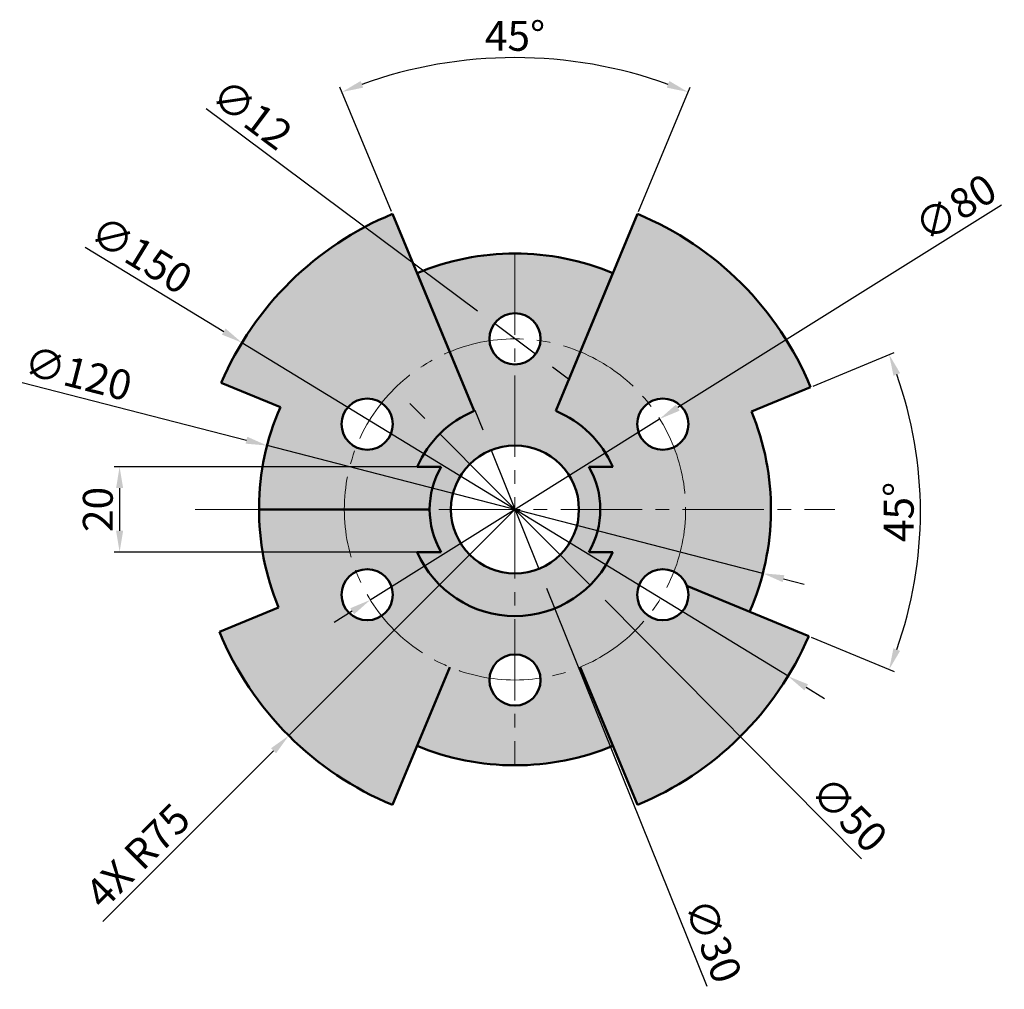
# Model space of a CAD drawing. Units: millimetres. Extents: x 3137 to 3368, y 1633 to 1861.
import ezdxf

# ---------------------------------------------------------------- set-up
doc = ezdxf.new("R2010")
doc.units = ezdxf.units.MM
doc.linetypes.add('CENTER2', pattern=[28.575, 19.05, -3.175, 3.175, -3.175])
for name, color, linetype, lineweight in [('M-CNTR', 1, 'CENTER2', 18), ('M-DIMS', 2, 'Continuous', 25), ('M-HATC', 252, 'Continuous', 18), ('M-OUTL', 7, 'Continuous', 50)]:
    doc.layers.add(name, color=color, linetype=linetype, lineweight=lineweight)
doc.styles.get("Standard").update_dxf_attribs({"font": 'arial.ttf'})
doc.dimstyles.new('ISO-25', dxfattribs={"dimtxt": 7, "dimasz": 5, "dimexe": 1.25, "dimexo": 0.625, "dimtad": 1, "dimtxsty": 'Standard', "dimcen": 2.5, "dimadec": 0, "dimazin": 0, "dimtfac": 1, "dimtmove": 0, "dimatfit": 3, "dimfxl": 1, "dimarcsym": 0})

# ---------------------------------------------------------------- blocks, each defined once
blk = doc.blocks.new('*D1')
at = {"layer": 'Defpoints', "color": 0, "transparency": 16777216}
for p in [(3267.36, 1850.91), (3224.83, 1815.15), (3282.23, 1815.15), (3243.97, 1768.96), (3263.1, 1768.96)]:
    blk.add_point(p, dxfattribs=at)
at = {"layer": 'M-DIMS', "color": 0, "lineweight": -2, "transparency": 16777216}
for p, q in [((3224.59, 1815.73), (3212.51, 1844.9)), ((3282.47, 1815.73), (3294.56, 1844.9))]:
    blk.add_line(p, q, dxfattribs=at)
blk.add_arc((3253.53, 1745.86), 105.95, 70.2042, 109.7958, dxfattribs=at)
at = {"layer": 'M-DIMS', "color": 0, "transparency": 16777216}
for points in [[(3217.95, 1844.77), (3217.35, 1846.33), (3212.99, 1843.75)], [(3289.71, 1846.33), (3289.11, 1844.77), (3294.08, 1843.75)]]:
    blk.add_solid(points, dxfattribs=at)
at = {"layer": 'M-DIMS', "color": 0, "transparency": 16777216, "insert": (3253.53, 1856), "char_height": 7, "attachment_point": 5}
blk.add_mtext('45°', dxfattribs=at)
blk = doc.blocks.new('*D2')
at = {"layer": 'Defpoints', "color": 0, "transparency": 16777216}
for p in [(3322.82, 1774.56), (3308.97, 1768.82), (3347.75, 1732.67), (3293.78, 1727.99), (3322.39, 1716.14)]:
    blk.add_point(p, dxfattribs=at)
at = {"layer": 'M-DIMS', "color": 0, "lineweight": -2, "transparency": 16777216}
for p, q in [((3323.4, 1774.8), (3342.38, 1782.67)), ((3322.97, 1715.9), (3342.38, 1707.86))]:
    blk.add_line(p, q, dxfattribs=at)
blk.add_arc((3252.08, 1745.26), 96.49, 340.4692, 19.5308, dxfattribs=at)
at = {"layer": 'M-DIMS', "color": 0, "transparency": 16777216}
for points in [[(3342.24, 1777.22), (3343.8, 1777.82), (3341.23, 1782.19)], [(3343.8, 1712.7), (3342.24, 1713.3), (3341.23, 1708.34)]]:
    blk.add_solid(points, dxfattribs=at)
at = {"layer": 'M-DIMS', "color": 0, "transparency": 16777216, "insert": (3344.39, 1745.26), "char_height": 7, "attachment_point": 5, "rotation": 90}
blk.add_mtext('45°', dxfattribs=at)
blk = doc.blocks.new('*D3')
at = {"layer": 'Defpoints', "color": 0, "transparency": 16777216}
for p in [(3233.42, 1755.86), (3160.86, 1735.86), (3233.42, 1735.86)]:
    blk.add_point(p, dxfattribs=at)
at = {"layer": 'M-DIMS', "color": 0, "lineweight": -2, "transparency": 16777216}
for p, q in [((3232.79, 1755.86), (3159.61, 1755.86)), ((3160.86, 1750.86), (3160.86, 1740.86)), ((3232.79, 1735.86), (3159.61, 1735.86))]:
    blk.add_line(p, q, dxfattribs=at)
at = {"layer": 'M-DIMS', "color": 0, "transparency": 16777216}
for points in [[(3160.03, 1750.86), (3161.69, 1750.86), (3160.86, 1755.86)], [(3160.03, 1740.86), (3161.69, 1740.86), (3160.86, 1735.86)]]:
    blk.add_solid(points, dxfattribs=at)
at = {"layer": 'M-DIMS', "color": 0, "transparency": 16777216, "insert": (3156.66, 1745.86), "char_height": 7, "attachment_point": 5, "rotation": 90}
blk.add_mtext('20', dxfattribs=at)
blk = doc.blocks.new('*D4')
at = {"layer": 'Defpoints', "color": 0, "transparency": 16777216}
for p in [(3189.53, 1784.97), (3317.53, 1706.76)]:
    blk.add_point(p, dxfattribs=at)
at = {"layer": 'M-DIMS', "color": 0, "lineweight": -2, "transparency": 16777216}
for p, q in [((3152.82, 1807.39), (3185.27, 1787.57)), ((3317.53, 1706.76), (3189.53, 1784.97)), ((3321.8, 1704.15), (3326.07, 1701.55))]:
    blk.add_line(p, q, dxfattribs=at)
at = {"layer": 'M-DIMS', "color": 0, "transparency": 16777216}
for points in [[(3185.7, 1788.28), (3184.83, 1786.86), (3189.53, 1784.97)], [(3322.23, 1704.86), (3321.36, 1703.44), (3317.53, 1706.76)]]:
    blk.add_solid(points, dxfattribs=at)
at = {"layer": 'M-DIMS', "color": 0, "transparency": 16777216, "insert": (3165.49, 1804.81), "char_height": 7, "attachment_point": 5, "rotation": 328.5759}
blk.add_mtext('∅150', dxfattribs=at)
blk = doc.blocks.new('*D5')
at = {"layer": 'Defpoints', "color": 0, "transparency": 16777216}
for p in [(3195.43, 1760.85), (3311.63, 1730.88)]:
    blk.add_point(p, dxfattribs=at)
at = {"layer": 'M-DIMS', "color": 0, "lineweight": -2, "transparency": 16777216}
for p, q in [((3138.04, 1775.65), (3190.59, 1762.1)), ((3311.63, 1730.88), (3195.43, 1760.85)), ((3316.47, 1729.63), (3321.31, 1728.38))]:
    blk.add_line(p, q, dxfattribs=at)
at = {"layer": 'M-DIMS', "color": 0, "transparency": 16777216}
for points in [[(3190.8, 1762.9), (3190.38, 1761.29), (3195.43, 1760.85)], [(3316.68, 1730.44), (3316.26, 1728.82), (3311.63, 1730.88)]]:
    blk.add_solid(points, dxfattribs=at)
at = {"layer": 'M-DIMS', "color": 0, "transparency": 16777216, "insert": (3150.91, 1776.87), "char_height": 7, "attachment_point": 5, "rotation": 345.5374}
blk.add_mtext('∅120', dxfattribs=at)
blk = doc.blocks.new('*D6')
at = {"layer": 'Defpoints', "color": 0, "transparency": 16777216}
for p in [(3287.44, 1767.08), (3219.62, 1724.65)]:
    blk.add_point(p, dxfattribs=at)
at = {"layer": 'M-DIMS', "color": 0, "lineweight": -2, "transparency": 16777216}
for p, q in [((3367.57, 1817.21), (3291.68, 1769.73)), ((3219.62, 1724.65), (3287.44, 1767.08)), ((3215.38, 1722), (3211.14, 1719.34))]:
    blk.add_line(p, q, dxfattribs=at)
at = {"layer": 'M-DIMS', "color": 0, "transparency": 16777216}
for points in [[(3291.24, 1770.44), (3292.12, 1769.02), (3287.44, 1767.08)], [(3214.94, 1722.7), (3215.83, 1721.29), (3219.62, 1724.65)]]:
    blk.add_solid(points, dxfattribs=at)
at = {"layer": 'M-DIMS', "color": 0, "transparency": 16777216, "insert": (3357.25, 1815.93), "char_height": 7, "attachment_point": 5, "rotation": 32.0318}
blk.add_mtext('∅80', dxfattribs=at)
blk = doc.blocks.new('*D7')
at = {"layer": 'Defpoints', "color": 0, "transparency": 16777216}
for p in [(3235.93, 1763.61), (3271.14, 1728.11)]:
    blk.add_point(p, dxfattribs=at)
at = {"layer": 'M-DIMS', "color": 0, "lineweight": -2, "transparency": 16777216}
for p, q in [((3232.41, 1767.16), (3228.89, 1770.71)), ((3235.93, 1763.61), (3271.14, 1728.11)), ((3334.75, 1663.97), (3274.66, 1724.56))]:
    blk.add_line(p, q, dxfattribs=at)
at = {"layer": 'M-DIMS', "color": 0, "transparency": 16777216}
for points in [[(3233, 1767.75), (3231.82, 1766.58), (3235.93, 1763.61)], [(3275.25, 1725.15), (3274.07, 1723.98), (3271.14, 1728.11)]]:
    blk.add_solid(points, dxfattribs=at)
at = {"layer": 'M-DIMS', "color": 0, "transparency": 16777216, "insert": (3331.22, 1673.77), "char_height": 7, "attachment_point": 5, "rotation": 314.7625}
blk.add_mtext('∅50', dxfattribs=at)
blk = doc.blocks.new('*D8')
at = {"layer": 'Defpoints', "color": 0, "transparency": 16777216}
for p in [(3247.93, 1759.78), (3259.14, 1731.95)]:
    blk.add_point(p, dxfattribs=at)
at = {"layer": 'M-DIMS', "color": 0, "lineweight": -2, "transparency": 16777216}
for p, q in [((3246.06, 1764.42), (3244.19, 1769.05)), ((3247.93, 1759.78), (3259.14, 1731.95)), ((3298.58, 1634), (3261, 1727.31))]:
    blk.add_line(p, q, dxfattribs=at)
at = {"layer": 'M-DIMS', "color": 0, "transparency": 16777216}
for points in [[(3246.83, 1764.73), (3245.29, 1764.1), (3247.93, 1759.78)], [(3261.78, 1727.62), (3260.23, 1727), (3259.14, 1731.95)]]:
    blk.add_solid(points, dxfattribs=at)
at = {"layer": 'M-DIMS', "color": 0, "transparency": 16777216, "insert": (3299.13, 1644.4), "char_height": 7, "attachment_point": 5, "rotation": 291.9338}
blk.add_mtext('∅30', dxfattribs=at)
blk = doc.blocks.new('*D9')
at = {"layer": 'Defpoints', "color": 0, "transparency": 16777216}
for p in [(3248.73, 1789.45), (3258.34, 1782.27)]:
    blk.add_point(p, dxfattribs=at)
at = {"layer": 'M-DIMS', "color": 0, "lineweight": -2, "transparency": 16777216}
for p, q in [((3181.17, 1839.91), (3244.72, 1792.45)), ((3258.34, 1782.27), (3248.73, 1789.45)), ((3262.35, 1779.28), (3266.35, 1776.29))]:
    blk.add_line(p, q, dxfattribs=at)
at = {"layer": 'M-DIMS', "color": 0, "transparency": 16777216}
for points in [[(3245.22, 1793.11), (3244.22, 1791.78), (3248.73, 1789.45)], [(3262.84, 1779.95), (3261.85, 1778.61), (3258.34, 1782.27)]]:
    blk.add_solid(points, dxfattribs=at)
at = {"layer": 'M-DIMS', "color": 0, "transparency": 16777216, "insert": (3191.34, 1837.8), "char_height": 7, "attachment_point": 5, "rotation": 323.2445}
blk.add_mtext('∅12', dxfattribs=at)
blk = doc.blocks.new('HOLE-D12')
blk.add_circle((6, 6), 6)
blk = doc.blocks.new('*D11')
at = {"layer": 'Defpoints', "color": 0, "transparency": 16777216}
for p in [(3253.53, 1745.86), (3200.5, 1692.83)]:
    blk.add_point(p, dxfattribs=at)
at = {"layer": 'M-DIMS', "color": 0, "lineweight": -2, "transparency": 16777216}
for p, q in [((3253.53, 1745.86), (3200.5, 1692.83)), ((3156.89, 1649.22), (3196.96, 1689.29))]:
    blk.add_line(p, q, dxfattribs=at)
at = {"layer": 'M-DIMS', "color": 0, "transparency": 16777216}
blk.add_solid([(3196.37, 1689.88), (3197.55, 1688.71), (3200.5, 1692.83)], dxfattribs=at)
at = {"layer": 'M-DIMS', "color": 0, "transparency": 16777216, "insert": (3165.72, 1663.97), "char_height": 7, "attachment_point": 5, "rotation": 44.9999}
blk.add_mtext('4X R75', dxfattribs=at)

msp = doc.modelspace()

# ---------------------------------------------------------------- hatches: boundary and pattern name
at = {"layer": 'M-HATC'}
h = msp.add_hatch(color=256, dxfattribs=at)
h.set_gradient(color1=(255, 255, 0), color2=(0, 255, 0), tint=1)
h.paths.add_polyline_path([(3224.831, 1815.154, 0.1950659), (3184.674, 1775.587), (3198.534, 1769.846, 0.1031671), (3193.532, 1745.863), (3213.532, 1745.863, -0.0936367), (3216.289, 1760.457, -0.2881683), (3212.891, 1765.863, -0.6026509), (3222.273, 1770.82, -0.1267619), (3238.225, 1782.818)])
h.paths.add_polyline_path([(3212.891, 1725.863, -0.2881683), (3216.289, 1731.27, -0.0936367), (3213.532, 1745.863), (3193.532, 1745.863, 0.0984914), (3198.1, 1722.902), (3184.241, 1717.162, 0.1989124), (3224.831, 1676.572), (3238.225, 1708.908, -0.1267619), (3222.273, 1720.907, -0.6026509)])
h.paths.add_polyline_path([(3233.532, 1745.863), (3213.532, 1745.863, 0.0936367), (3216.289, 1731.27, -0.5525921), (3224.891, 1725.863, -0.2479324), (3222.273, 1720.907, 0.1267619), (3238.225, 1708.908, 0.060714), (3247.549, 1706.313, -0.392393), (3253.532, 1711.863), (3253.532, 1720.863, -0.2982166), (3230.619, 1735.863), (3236.212, 1735.863, -0.1316525)])
h.paths.add_polyline_path([(3243.965, 1768.96), (3238.225, 1782.818, 0.1267619), (3222.273, 1770.82, -0.2479324), (3224.891, 1765.863, -0.5525921), (3216.289, 1760.457, 0.0936367), (3213.532, 1745.863), (3233.532, 1745.863, -0.1316525), (3236.212, 1755.863), (3230.619, 1755.863, -0.1940263)])
h = msp.add_hatch(color=256, dxfattribs=at)
h.set_gradient(color1=(0, 255, 255), color2=(0, 255, 255), tint=1, name='INVCYLINDER')
h.paths.add_polyline_path([(3282.234, 1815.154), (3268.84, 1782.818, -0.1267619), (3284.792, 1770.82, -0.6026509), (3294.173, 1765.863, -0.2881683), (3290.775, 1760.457, -0.0936367), (3293.532, 1745.863), (3313.532, 1745.863, 0.0984914), (3308.965, 1768.824), (3322.823, 1774.564, 0.1989124)])
h.paths.add_polyline_path([(3313.532, 1745.863), (3293.532, 1745.863, -0.0936367), (3290.775, 1731.27, -0.1923993), (3293.785, 1727.988), (3308.53, 1721.88, 0.1031671)])
h.paths.add_polyline_path([(3322.391, 1716.139), (3293.785, 1727.988, -0.0907382), (3294.173, 1725.863, -0.6026509), (3284.792, 1720.907, -0.1267619), (3268.84, 1708.908), (3282.234, 1676.572, 0.1950659)])
h = msp.add_hatch(color=256, dxfattribs=at)
h.set_gradient(color1=(0, 0, 255), tint=1, name='INVCYLINDER')
h.paths.add_polyline_path([(3253.532, 1791.863), (3253.532, 1805.863, 0.0984914), (3230.571, 1801.296), (3238.225, 1782.818, -0.060714), (3247.549, 1785.413, -0.0187698), (3247.532, 1785.863, -0.4142136)])
h.paths.add_polyline_path([(3276.493, 1801.296, 0.0984914), (3253.532, 1805.863), (3253.532, 1791.863, -0.4363761), (3259.515, 1785.413, -0.060714), (3268.84, 1782.818)])
h.paths.add_polyline_path([(3268.84, 1782.818, 0.060714), (3259.515, 1785.413, -0.392393), (3253.532, 1779.863), (3253.532, 1760.863, -0.4142136), (3268.532, 1745.863), (3273.532, 1745.863, 0.1316525), (3270.853, 1755.863), (3276.445, 1755.863, 0.1940263), (3263.099, 1768.96)])
h.paths.add_polyline_path([(3253.532, 1779.863, -0.392393), (3247.549, 1785.413, 0.060714), (3238.225, 1782.818), (3243.965, 1768.96, 0.1940263), (3230.619, 1755.863), (3236.212, 1755.863, 0.1316525), (3233.532, 1745.863), (3238.532, 1745.863, -0.4142136), (3253.532, 1760.863)])
h.paths.add_polyline_path([(3238.532, 1745.863), (3233.532, 1745.863, 0.1316525), (3236.212, 1735.863), (3230.619, 1735.863, 0.2982166), (3253.532, 1720.863), (3253.532, 1730.863, -0.4142136)])
h.paths.add_polyline_path([(3276.445, 1735.863), (3270.853, 1735.863, 0.1316525), (3273.532, 1745.863), (3268.532, 1745.863, -0.4142136), (3253.532, 1730.863), (3253.532, 1720.863, 0.2982166)], flags=17)
h.paths.add_polyline_path([(3284.792, 1720.907, -0.2479324), (3282.173, 1725.863, -0.5525921), (3290.775, 1731.27, 0.0936367), (3293.532, 1745.863), (3273.532, 1745.863, -0.1316525), (3270.853, 1735.863), (3276.445, 1735.863, -0.2982166), (3253.532, 1720.863), (3253.532, 1711.863, -0.392393), (3259.515, 1706.313, 0.1889299)])
h.paths.add_polyline_path([(3290.775, 1760.457, -0.5525921), (3282.173, 1765.863, -0.2479324), (3284.792, 1770.82, 0.1267619), (3268.84, 1782.818), (3263.099, 1768.96, -0.1940263), (3276.445, 1755.863), (3270.853, 1755.863, -0.1316525), (3273.532, 1745.863), (3293.532, 1745.863, 0.0936367)])
h.paths.add_polyline_path([(3268.84, 1708.908, -0.060714), (3259.515, 1706.313, -0.0187698), (3259.532, 1705.863, -0.4142136), (3253.532, 1699.863), (3253.532, 1685.863, 0.0984914), (3276.493, 1690.43)])
h.paths.add_polyline_path([(3253.532, 1699.863, -0.4363761), (3247.549, 1706.313, -0.060714), (3238.225, 1708.908), (3230.571, 1690.43, 0.0984914), (3253.532, 1685.863)])

# ---------------------------------------------------------------- linework, layer by layer
at = {"layer": 'M-CNTR'}
for p, q in [((3253.532, 1805.863), (3253.532, 1685.863)), ((3178.532, 1745.863), (3328.532, 1745.863))]:
    msp.add_line(p, q, dxfattribs=at)
msp.add_circle((3253.532, 1745.863), 40, dxfattribs=at)
at = {"layer": 'M-OUTL'}
for p, q in [((3243.965, 1768.96), (3224.831, 1815.154)), ((3263.099, 1768.96), (3282.234, 1815.154)), ((3243.965, 1768.96), (3230.571, 1801.296)), ((3263.099, 1768.96), (3276.493, 1801.296)), ((3198.534, 1769.846), (3184.674, 1775.587)), ((3308.965, 1768.824), (3322.823, 1774.564)), ((3236.212, 1755.863), (3230.619, 1755.863)), ((3276.445, 1755.863), (3270.853, 1755.863)), ((3233.532, 1745.863), (3193.532, 1745.863)), ((3236.212, 1735.863), (3230.619, 1735.863)), ((3276.445, 1735.863), (3270.853, 1735.863)), ((3293.785, 1727.988), (3322.391, 1716.139)), ((3198.1, 1722.902), (3184.241, 1717.162)), ((3238.225, 1708.908), (3224.831, 1676.572)), ((3268.84, 1708.908), (3282.234, 1676.572))]:
    msp.add_line(p, q, dxfattribs=at)
msp.add_circle((3253.532, 1745.863), 15, dxfattribs=at)
for radius, start, end in [(75, 112.5, 156.65138), (75, 22.5, 67.5), (60, 67.5, 112.5), (60, 156.43921, 202.5), (25, 112.5, 156.42182), (25, 23.57818, 67.5), (60, 336.43921, 22.5), (20, 150, 210), (20, 330, 30), (25, 203.57818, 336.42182), (75, 202.5, 247.5), (75, 292.5, 336.65138), (60, 247.5, 292.5)]:
    msp.add_arc((3253.532, 1745.863), radius, start, end, dxfattribs=at)

# ---------------------------------------------------------------- block references
for p in [(3247.532, 1779.863), (3212.891, 1759.863), (3282.173, 1759.863), (3212.891, 1719.863), (3282.173, 1719.863), (3247.532, 1699.863)]:
    msp.add_blockref('HOLE-D12', p, dxfattribs=at)

# ---------------------------------------------------------------- dimensions: what is measured, and where the dimension line sits
at = {"layer": 'M-DIMS'}
for base, line1, line2, picture, middle in [((3267.361, 1850.906), ((3263.099, 1768.96), (3282.234, 1815.154)), ((3243.965, 1768.96), (3224.831, 1815.154)), '*D1', (3253.532, 1855.997)), ((3347.748, 1732.667), ((3293.785, 1727.988), (3322.391, 1716.139)), ((3308.965, 1768.824), (3322.823, 1774.564)), '*D2', (3344.389, 1745.262))]:
    dim = msp.add_angular_dim_2l(base=base, line1=line1, line2=line2, dimstyle='ISO-25', override={"dimclrd": 0, "dimclre": 0, "dimclrt": 0}, dxfattribs=at)
    dim.commit()
    dim.dimension.update_dxf_attribs({"geometry": picture, "text_midpoint": middle})
for p1, p2, picture, middle in [((3258.339, 1782.273), (3248.725, 1789.453), '*D9', (3188.711, 1834.277)), ((3219.622, 1724.647), (3287.442, 1767.079), '*D6', (3359.577, 1812.209)), ((3317.532, 1706.76), (3189.532, 1784.966), '*D4', (3163.195, 1801.057)), ((3311.631, 1730.878), (3195.434, 1760.848), '*D5', (3149.813, 1772.614)), ((3235.928, 1763.614), (3271.137, 1728.112), '*D7', (3328.102, 1670.673)), ((3247.929, 1759.777), (3259.135, 1731.949), '*D8', (3295.052, 1642.756))]:
    dim = msp.add_diameter_dim_2p(p1=p1, p2=p2, dimstyle='ISO-25', override={"dimclrd": 0, "dimclre": 0, "dimclrt": 0}, dxfattribs=at)
    dim.commit()
    dim.dimension.update_dxf_attribs({"geometry": picture, "text_midpoint": middle, "dimtype": 163})
dim = msp.add_linear_dim(base=(3160.859, 1735.863), p1=(3233.416, 1755.863), p2=(3233.416, 1735.863), angle=90, dimstyle='ISO-25', override={"dimclrd": 0, "dimclre": 0, "dimclrt": 0}, dxfattribs=at)
dim.commit()
dim.dimension.update_dxf_attribs({"geometry": '*D3', "text_midpoint": (3156.66, 1745.863)})
dim = msp.add_radius_dim(center=(3253.532, 1745.863), mpoint=(3200.499, 1692.83), text='4X <>', dimstyle='ISO-25', override={"dimdec": 0, "dimlfac": 1, "dimrnd": 0, "dimzin": 0, "dimdsep": 46, "dimlunit": 2}, dxfattribs=at)
dim.commit()
dim.dimension.update_dxf_attribs({"geometry": '*D11', "text_midpoint": (3168.679, 1661.01), "dimtype": 164})

doc.saveas('drawing.dxf')
